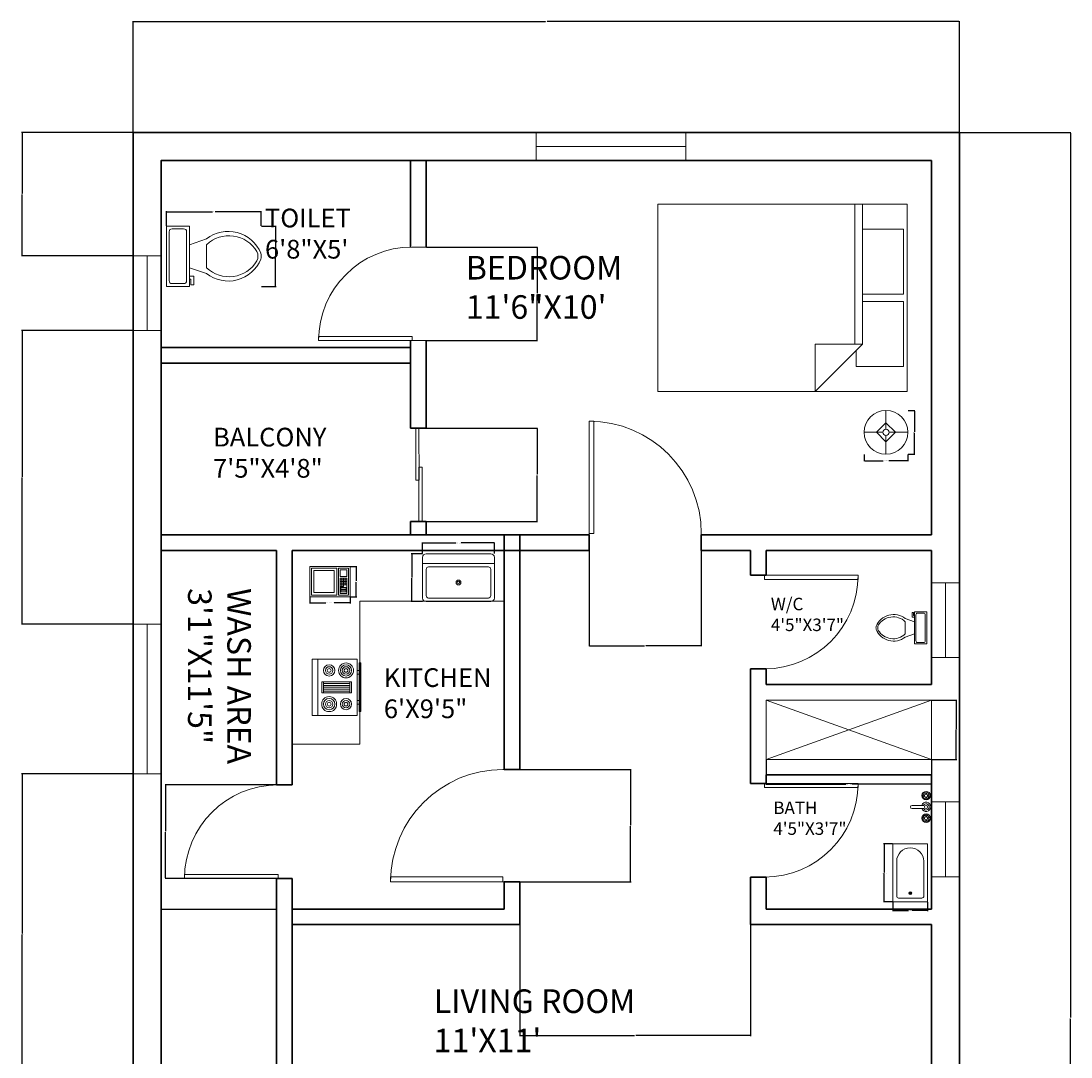
# Model space of a CAD drawing. Units: inches. Extents: x 7766 to 8631, y 9203 to 9940.
# Tile 6 of 6: x 8294 to 8631, y 9608 to 9940. Entities that reach past the tile are written whole.
import ezdxf

# ---------------------------------------------------------------- set-up
doc = ezdxf.new("R2010")
doc.units = ezdxf.units.IN
for name, color, linetype, lineweight in [('A-ANNO-DIMS', 2, 'Continuous', 18), ('A-AREA-IDEN', 11, 'Continuous', 18), ('A-EQPM', 9, 'Continuous', 18), ('A-FLOR-CASE', 7, 'Continuous', 20), ('A-FLOR-FIXT', 9, 'Continuous', 18), ('A-FLOR-OPEN', 7, 'Continuous', 18), ('A-WALL', 7, 'Continuous', 35), ('door', 1, 'Continuous', 18), ('floor', 7, 'Continuous', 25), ('furniture', 6, 'Continuous', 18), ('window', 3, 'Continuous', 18)]:
    doc.layers.add(name, color=color, linetype=linetype, lineweight=lineweight)
doc.styles.get("Standard").update_dxf_attribs({"font": 'arial.ttf'})
doc.dimstyles.get("Standard").update_dxf_attribs({"dimtxt": 0.18, "dimasz": 0.18, "dimexe": 0.18, "dimexo": 0.0625, "dimgap": 0.09, "dimtad": 0, "dimtih": 1, "dimtoh": 1, "dimdec": 4, "dimzin": 0, "dimdsep": 46, "dimtxsty": 'Standard', "dimcen": 0.09, "dimadec": 0, "dimazin": 0, "dimtfac": 1, "dimtdec": 4, "dimtofl": 0, "dimtmove": 0, "dimatfit": 3, "dimfxl": 1, "dimtolj": 1, "dimtzin": 0, "dimarcsym": 0})

# ---------------------------------------------------------------- blocks, each defined once
blk = doc.blocks.new('*U2')
for p, q in [((0, 0), (0, -6)), ((40, 0), (40, -6))]:
    blk.add_line(p, q)
blk.add_lwpolyline([(0, 0), (0, 40), (1.75, 40), (1.75, 0)], close=True)
blk.add_arc((0, 0), 40, 0, 90)
blk = doc.blocks.new('*U4')
for p, q in [((0, 0), (0, -6)), ((40, 0), (40, -6))]:
    blk.add_line(p, q)
blk.add_lwpolyline([(0, 0), (0, 40), (1.75, 40), (1.75, 0)], close=True)
blk.add_arc((0, 0), 40, 0, 90)
blk = doc.blocks.new('Bed - Queen')
for p, q in [((0, -80.00003), (0, 0)), ((0, 0), (59.99999, 0)), ((59.99999, 0), (59.99999, -80.00003)), ((7.99999, -1.2), (28.79998, -1.2)), ((7.99999, -14.4), (7.99999, -1.2)), ((28.79998, -1.2), (28.79998, -14.4)), ((31.19999, -1.2), (51.99999, -1.2)), ((31.19999, -14.4), (31.19999, -1.2)), ((51.99999, -1.2), (51.99999, -16.4)), ((0, -14.4), (44.8, -14.4)), ((44.8, -16.8), (0, -16.8)), ((59.99999, -29.6), (44.8, -14.4)), ((44.8, -14.4), (44.8, -29.6)), ((51.99999, -16.4), (46.79936, -16.4)), ((44.8, -29.6), (59.99999, -29.6)), ((59.99999, -80.00003), (0, -80.00003))]:
    blk.add_line(p, q)
blk = doc.blocks.new('Microwave')
for p, q in [((18, 10), (22, 10)), ((22, 9), (18, 9)), ((18, 8), (22, 8)), ((22, 7), (18, 7)), ((19, 7), (19, 11)), ((19, 6), (19, 7)), ((20, 11), (20, 7)), ((20, 7), (20, 6)), ((21, 7), (21, 11)), ((20, 6), (18, 6))]:
    blk.add_line(p, q)
for points in [[(0, 0), (0, 18), (24, 18), (24, 0)], [(1, 1), (1, 17), (16, 17), (16, 1)], [(2.5, 2.5), (2.5, 15.5), (14.5, 15.5), (14.5, 2.5)], [(17, 1), (17, 17), (23, 17), (23, 1)], [(18, 12), (18, 16), (22, 16), (22, 12)], [(18, 2), (18, 11), (22, 11), (22, 2)], [(18.5, 4.5), (18.5, 5.5), (21.5, 5.5), (21.5, 4.5)], [(18.5, 3), (18.5, 4), (21.5, 4), (21.5, 3)]]:
    blk.add_lwpolyline(points, close=True)
blk = doc.blocks.new('Range-Oven - 30 in top')
for p, q in [((0, -3), (30, -3)), ((12, -6), (18, -6)), ((13, -20), (13, -6)), ((14, -6), (14, -20)), ((15, -20), (15, -6)), ((16, -6), (16, -20)), ((17, -20), (17, -6)), ((18, -20), (12, -20)), ((6, -24), (6, -25)), ((8, -25), (8, -24)), ((22, -25), (22, -24)), ((24, -24), (24, -25))]:
    blk.add_line(p, q)
for points in [[(0, -24), (0, 0), (30, 0), (30, -24)], [(12, -21), (12, -5), (18, -5), (18, -21)], [(2, -26), (2, -25), (28, -25), (28, -26)]]:
    blk.add_lwpolyline(points, close=True)
for centre, radius in [((6, -9), 4), ((6, -9), 3), ((6, -9), 2), ((6, -9), 1), ((24, -9), 3), ((24, -9), 2), ((24, -9), 1), ((6, -18), 3), ((6, -18), 2), ((24, -18), 4), ((24, -18), 3), ((24, -18), 2), ((6, -18), 1), ((24, -18), 1)]:
    blk.add_circle(centre, radius)
blk = doc.blocks.new('Sink-single - 30 in top')
blk.add_line((-15, -3.999996), (15, -3.999996))
for points in [[(-13.5, 0), (13.5, 0)], [(-15, -18.499996), (-15, -1.5)], [(15, -1.5), (15, -18.499996)], [(-13.5, -17.499996), (-13.5, -6.499996)], [(-12.5, -5.499996), (12.5, -5.499996)], [(13.5, -6.499996), (13.5, -17.499996)], [(13.5, -19.999996), (-13.5, -19.999996)], [(12.5, -18.499996), (-12.5, -18.499996)]]:
    blk.add_lwpolyline(points)
for radius in [1, 0.5]:
    blk.add_circle((0, -11.999996), radius)
for centre, radius, start, end in [((-13.5, -1.5), 1.5, 90, 180), ((13.5, -1.5), 1.5, 0, 90), ((-12.5, -6.499996), 1, 90, 180), ((12.5, -6.499996), 1, 0, 90), ((-12.5, -17.499996), 1, 180, 270), ((12.5, -17.499996), 1, 270, 0), ((-13.5, -18.499996), 1.5, 180, 270), ((13.5, -18.499996), 1.5, 270, 0)]:
    blk.add_arc(centre, radius, start, end)
blk = doc.blocks.new('Lamp - Table')
for p, q in [((0, 7), (0, 1)), ((-1, 0), (-7, 0)), ((0, 3), (-3, 0)), ((-3, 0), (0, -3)), ((3, 0), (0, 3)), ((0, -3), (3, 0)), ((1, 0), (7, 0)), ((0, -1), (0, -7))]:
    blk.add_line(p, q)
for radius in [7, 1]:
    blk.add_circle((0, 0), radius)
blk = doc.blocks.new('Toilet - top')
for p, q in [((9.5, -6), (9.5, -2)), ((-10, -8.5), (-8, -8.5)), ((-10, -9.5), (-10, -8.5)), ((-7, -9.5), (-10, -9.5)), ((-8, -8.5), (-8, -8)), ((-7, -8), (-7, -9.5)), ((-4, -8), (-6, -14)), ((4, -8), (6, -14)), ((4, -14), (-4, -14))]:
    blk.add_line(p, q)
blk.add_lwpolyline([(10.5, -8), (10.5, 0), (-10.5, 0), (-10.5, -8)], close=True)
for points in [[(-9.5, -2), (-9.5, -6)], [(8.5, -1), (-8.5, -1)], [(-8.5, -7), (8.5, -7)]]:
    blk.add_lwpolyline(points)
for centre, radius, start, end in [((-8.62, -1.88), 0.884, 81.8699, 188.1301), ((8.62, -1.88), 0.884, 351.8699, 98.1301), ((-8.62, -6.12), 0.884, 171.8699, 278.1301), ((8.62, -6.12), 0.884, 261.8699, 8.1301), ((3.52, -21.58), 12.17, 141.4691, 247.9714), ((4.2, -21.82), 11.33, 136.3677, 238.9468), ((-3.52, -21.58), 12.17, 292.0284, 38.5307), ((-4.2, -21.82), 11.33, 301.053, 43.6321), ((0, -27.88), 4, 245.7318, 294.2682), ((0, -29), 4, 254.8605, 285.1395)]:
    blk.add_arc(centre, radius, start, end)
blk = doc.blocks.new('Faucet - Bathroom top')
for p, q in [((-4.107, 0.125), (-4.375, 0.125)), ((-3.75, 0.4788), (-3.75, 0.75)), ((-3.5, 0.482), (-3.5, 0.75)), ((-3.1461, 0.125), (-2.875, 0.125)), ((3.143, 0.125), (2.875, 0.125)), ((3.5, 0.4788), (3.5, 0.75)), ((3.75, 0.482), (3.75, 0.75)), ((4.1039, 0.125), (4.375, 0.125)), ((-4.1039, -0.125), (-4.375, -0.125)), ((-3.75, -0.4821), (-3.75, -0.75)), ((-3.5, -0.4789), (-3.5, -0.75)), ((-3.143, -0.125), (-2.875, -0.125)), ((-0.5, -0.8639), (-0.5, -4.5)), ((0.5, -4.5), (0.5, -0.8631)), ((3.1461, -0.125), (2.875, -0.125)), ((3.5, -0.4821), (3.5, -0.75)), ((3.75, -0.4789), (3.75, -0.75)), ((4.107, -0.125), (4.375, -0.125))]:
    blk.add_line(p, q)
for centre, radius in [((-3.625, 0), 1.375), ((-4.625, 0), 0.2795), ((-3.625, 0), 0.5), ((-3.625, 1), 0.2795), ((-2.625, 0), 0.2795), ((0, 0), 0.5), ((3.625, 0), 1.375), ((2.625, 0), 0.2795), ((3.625, 0), 0.5), ((3.625, 1), 0.2795), ((4.625, 0), 0.2795), ((-3.625, -1), 0.2795), ((3.625, -1), 0.2795)]:
    blk.add_circle(centre, radius)
for centre, radius, start, end in [((-3.625, 0), 1, 105.2407, 164.2093), ((-3.625, 0), 1, 16.44125, 74.07887), ((0, 0), 1.5, 289.6514, 250.3603), ((0, 0), 1, 300.3431, 239.7554), ((3.625, 0), 1, 106.12, 164.0884), ((3.625, 0), 1, 16.23422, 73.90469), ((-3.625, 0), 1, 196.2342, 253.9047), ((-3.625, 0), 1, 286.12, 344.0884), ((3.625, 0), 1, 196.4413, 254.0789), ((3.625, 0), 1, 285.2407, 344.2093), ((0, -4.5), 0.5, 180, 0)]:
    blk.add_arc(centre, radius, start, end)
blk = doc.blocks.new('Bath Tub - 26 x 60 in.')
for p, q in [((8, -18), (10, -18)), ((9, -17), (9, -19))]:
    blk.add_line(p, q)
blk.add_lwpolyline([(0, -36), (0, 0), (60, 0), (60, -36)], close=True)
for points in [[(4, -30), (4, -6)], [(6, -4), (42, -4)], [(42, -32), (6, -32)]]:
    blk.add_lwpolyline(points)
for radius in [1.5, 1]:
    blk.add_circle((9, -18), radius)
for centre, radius, start, end in [((5.75, -5.75), 1.77, 81.8699, 188.1301), ((42, -18), 14, 270, 90), ((5.75, -30.25), 1.77, 171.8699, 278.1301)]:
    blk.add_arc(centre, radius, start, end)
blk = doc.blocks.new('WIN-48IN')
blk.add_line((4.5, 48), (4.5, 0))
blk.add_lwpolyline([(0, 48), (9, 48), (9, 0), (0, 0)], close=True)
blk = doc.blocks.new('WIN-24IN')
blk.add_line((4.5, 24), (4.5, 0))
blk.add_lwpolyline([(0, 24), (9, 24), (9, 0), (0, 0)], close=True)
blk = doc.blocks.new('COUNTER-L-KITCHEN')
for points in [[(21.71, 45.84), (68, 45.84), (68, 62.12), (0, 62.12), (0, 45.84)], [(21.71, 45.84), (21.71, 0), (0, 0), (0, 62.12), (21.71, 62.12)]]:
    blk.add_lwpolyline(points)
blk = doc.blocks.new('SHAFT-53X19')
for p, q in [((0, 19), (53, 19)), ((0, 0), (0, 19)), ((0, 19), (53, 0)), ((53, 19), (0, 0)), ((53, 0), (53, 19)), ((0, 0), (53, 0))]:
    blk.add_line(p, q)
blk = doc.blocks.new('*D34')
at = {"layer": 'A-ANNO-DIMS', "color": 0, "lineweight": -2, "transparency": 16777216}
for p, q in [((8340.53, 9874.62), (8340.53, 9879.3)), ((8340.71, 9879.12), (8355.28, 9879.12)), ((8370.78, 9879.12), (8356.21, 9879.12)), ((8370.96, 9874.62), (8370.96, 9879.3))]:
    blk.add_line(p, q, dxfattribs=at)
at = {"layer": 'A-ANNO-DIMS', "color": 0, "transparency": 16777216}
for points in [[(8340.71, 9879.15), (8340.71, 9879.09), (8340.53, 9879.12)], [(8370.78, 9879.15), (8370.78, 9879.09), (8370.96, 9879.12)]]:
    blk.add_solid(points, dxfattribs=at)
at = {"layer": 'Defpoints', "color": 0, "transparency": 16777216}
for p in [(8340.53, 9879.12), (8340.53, 9874.55), (8370.96, 9874.55)]:
    blk.add_point(p, dxfattribs=at)
at = {"layer": 'A-ANNO-DIMS', "color": 0, "transparency": 16777216, "insert": (8355.75, 9879.12), "char_height": 0.18, "attachment_point": 5}
blk.add_mtext('\\A1;WC 30', dxfattribs=at)
blk = doc.blocks.new('*D35')
at = {"layer": 'A-ANNO-DIMS', "color": 0, "lineweight": -2, "transparency": 16777216}
for p, q in [((8371.03, 9874.55), (8375.71, 9874.55)), ((8375.53, 9874.37), (8375.53, 9865.07)), ((8375.53, 9855.39), (8375.53, 9864.7)), ((8371.03, 9855.21), (8375.71, 9855.21))]:
    blk.add_line(p, q, dxfattribs=at)
at = {"layer": 'A-ANNO-DIMS', "color": 0, "transparency": 16777216}
for points in [[(8375.5, 9874.37), (8375.56, 9874.37), (8375.53, 9874.55)], [(8375.5, 9855.39), (8375.56, 9855.39), (8375.53, 9855.21)]]:
    blk.add_solid(points, dxfattribs=at)
at = {"layer": 'Defpoints', "color": 0, "transparency": 16777216}
for p in [(8370.96, 9874.55), (8375.53, 9874.55), (8370.96, 9855.21)]:
    blk.add_point(p, dxfattribs=at)
at = {"layer": 'A-ANNO-DIMS', "color": 0, "transparency": 16777216, "insert": (8375.53, 9864.88), "char_height": 0.18, "attachment_point": 5}
blk.add_mtext('\\A1;19', dxfattribs=at)
blk = doc.blocks.new('*D46')
at = {"layer": 'A-ANNO-DIMS', "color": 0, "lineweight": -2, "transparency": 16777216}
for p, q in [((8386.48, 9755.63), (8386.48, 9753.56)), ((8386.66, 9753.74), (8391.63, 9753.74)), ((8399.3, 9753.74), (8394.33, 9753.74)), ((8399.48, 9755.63), (8399.48, 9753.56))]:
    blk.add_line(p, q, dxfattribs=at)
at = {"layer": 'A-ANNO-DIMS', "color": 0, "transparency": 16777216}
for points in [[(8386.66, 9753.77), (8386.66, 9753.71), (8386.48, 9753.74)], [(8399.3, 9753.77), (8399.3, 9753.71), (8399.48, 9753.74)]]:
    blk.add_solid(points, dxfattribs=at)
at = {"layer": 'Defpoints', "color": 0, "transparency": 16777216}
for p in [(8386.48, 9755.69), (8399.48, 9755.69), (8399.48, 9753.74)]:
    blk.add_point(p, dxfattribs=at)
at = {"layer": 'A-ANNO-DIMS', "color": 0, "transparency": 16777216, "insert": (8392.98, 9753.74), "char_height": 0.18, "attachment_point": 5}
blk.add_mtext('\\A1;MICROWAVE 13 TYP.', dxfattribs=at)
blk = doc.blocks.new('*D47')
at = {"layer": 'A-ANNO-DIMS', "color": 0, "lineweight": -2, "transparency": 16777216}
for p, q in [((8399.54, 9765.44), (8401.61, 9765.44)), ((8401.43, 9765.26), (8401.43, 9760.75)), ((8401.43, 9755.87), (8401.43, 9760.38)), ((8399.54, 9755.69), (8401.61, 9755.69))]:
    blk.add_line(p, q, dxfattribs=at)
at = {"layer": 'A-ANNO-DIMS', "color": 0, "transparency": 16777216}
for points in [[(8401.4, 9765.26), (8401.46, 9765.26), (8401.43, 9765.44)], [(8401.4, 9755.87), (8401.46, 9755.87), (8401.43, 9755.69)]]:
    blk.add_solid(points, dxfattribs=at)
at = {"layer": 'Defpoints', "color": 0, "transparency": 16777216}
for p in [(8399.48, 9765.44), (8401.43, 9765.44), (8399.48, 9755.69)]:
    blk.add_point(p, dxfattribs=at)
at = {"layer": 'A-ANNO-DIMS', "color": 0, "transparency": 16777216, "insert": (8401.43, 9760.56), "char_height": 0.18, "attachment_point": 5}
blk.add_mtext('\\A1;10 TYP.', dxfattribs=at)
blk = doc.blocks.new('*D50')
at = {"layer": 'A-ANNO-DIMS', "color": 0, "lineweight": -2, "transparency": 16777216}
for p, q in [((8422.69, 9769.54), (8422.69, 9773.11)), ((8422.87, 9772.93), (8433.33, 9772.93)), ((8445.51, 9772.93), (8435.04, 9772.93)), ((8445.69, 9769.54), (8445.69, 9773.11))]:
    blk.add_line(p, q, dxfattribs=at)
at = {"layer": 'A-ANNO-DIMS', "color": 0, "transparency": 16777216}
for points in [[(8422.87, 9772.96), (8422.87, 9772.9), (8422.69, 9772.93)], [(8445.51, 9772.96), (8445.51, 9772.9), (8445.69, 9772.93)]]:
    blk.add_solid(points, dxfattribs=at)
at = {"layer": 'Defpoints', "color": 0, "transparency": 16777216}
for p in [(8445.69, 9772.93), (8422.69, 9769.48), (8445.69, 9769.48)]:
    blk.add_point(p, dxfattribs=at)
at = {"layer": 'A-ANNO-DIMS', "color": 0, "transparency": 16777216, "insert": (8434.19, 9772.93), "char_height": 0.18, "attachment_point": 5}
blk.add_mtext('\\A1;SINK 23 TYP.', dxfattribs=at)
blk = doc.blocks.new('*D51')
at = {"layer": 'A-ANNO-DIMS', "color": 0, "lineweight": -2, "transparency": 16777216}
for p, q in [((8422.62, 9769.48), (8419.06, 9769.48)), ((8419.24, 9769.3), (8419.24, 9761.99)), ((8419.24, 9754.32), (8419.24, 9761.63)), ((8422.62, 9754.14), (8419.06, 9754.14))]:
    blk.add_line(p, q, dxfattribs=at)
at = {"layer": 'A-ANNO-DIMS', "color": 0, "transparency": 16777216}
for points in [[(8419.21, 9769.3), (8419.27, 9769.3), (8419.24, 9769.48)], [(8419.21, 9754.32), (8419.27, 9754.32), (8419.24, 9754.14)]]:
    blk.add_solid(points, dxfattribs=at)
at = {"layer": 'Defpoints', "color": 0, "transparency": 16777216}
for p in [(8419.24, 9769.48), (8422.69, 9769.48), (8422.69, 9754.14)]:
    blk.add_point(p, dxfattribs=at)
at = {"layer": 'A-ANNO-DIMS', "color": 0, "transparency": 16777216, "insert": (8419.24, 9761.81), "char_height": 0.18, "attachment_point": 5}
blk.add_mtext('\\A1;15 TYP.', dxfattribs=at)
blk = doc.blocks.new('*D52')
at = {"layer": 'A-ANNO-DIMS', "color": 0, "lineweight": -2, "transparency": 16777216}
for p, q in [((8564.27, 9801.35), (8564.27, 9799.13)), ((8578.27, 9801.35), (8578.27, 9799.13)), ((8564.45, 9799.31), (8570.37, 9799.31)), ((8578.09, 9799.31), (8572.17, 9799.31))]:
    blk.add_line(p, q, dxfattribs=at)
at = {"layer": 'A-ANNO-DIMS', "color": 0, "transparency": 16777216}
for points in [[(8564.45, 9799.34), (8564.45, 9799.28), (8564.27, 9799.31)], [(8578.09, 9799.34), (8578.09, 9799.28), (8578.27, 9799.31)]]:
    blk.add_solid(points, dxfattribs=at)
at = {"layer": 'Defpoints', "color": 0, "transparency": 16777216}
for p in [(8564.27, 9801.41), (8578.27, 9801.41), (8578.27, 9799.31)]:
    blk.add_point(p, dxfattribs=at)
at = {"layer": 'A-ANNO-DIMS', "color": 0, "transparency": 16777216, "insert": (8571.27, 9799.31), "char_height": 0.18, "attachment_point": 5}
blk.add_mtext('\\A1;LAMP 14 TYP.', dxfattribs=at)
blk = doc.blocks.new('*D53')
at = {"layer": 'A-ANNO-DIMS', "color": 0, "lineweight": -2, "transparency": 16777216}
for p, q in [((8578.33, 9815.41), (8580.55, 9815.41)), ((8580.37, 9815.23), (8580.37, 9808.59)), ((8580.37, 9801.59), (8580.37, 9808.23)), ((8578.33, 9801.41), (8580.55, 9801.41))]:
    blk.add_line(p, q, dxfattribs=at)
at = {"layer": 'A-ANNO-DIMS', "color": 0, "transparency": 16777216}
for points in [[(8580.34, 9815.23), (8580.4, 9815.23), (8580.37, 9815.41)], [(8580.34, 9801.59), (8580.4, 9801.59), (8580.37, 9801.41)]]:
    blk.add_solid(points, dxfattribs=at)
at = {"layer": 'Defpoints', "color": 0, "transparency": 16777216}
for p in [(8578.27, 9815.41), (8580.37, 9815.41), (8578.27, 9801.41)]:
    blk.add_point(p, dxfattribs=at)
at = {"layer": 'A-ANNO-DIMS', "color": 0, "transparency": 16777216, "insert": (8580.37, 9808.41), "char_height": 0.18, "attachment_point": 5}
blk.add_mtext('\\A1;14 TYP.', dxfattribs=at)
blk = doc.blocks.new('*D56')
at = {"layer": 'A-ANNO-DIMS', "color": 0, "lineweight": -2, "transparency": 16777216}
for p, q in [((8573.4, 9676.45), (8570.49, 9676.45)), ((8570.67, 9676.27), (8570.67, 9667.33)), ((8570.67, 9658.03), (8570.67, 9666.97)), ((8573.4, 9657.85), (8570.49, 9657.85))]:
    blk.add_line(p, q, dxfattribs=at)
at = {"layer": 'A-ANNO-DIMS', "color": 0, "transparency": 16777216}
for points in [[(8570.64, 9676.27), (8570.7, 9676.27), (8570.67, 9676.45)], [(8570.64, 9658.03), (8570.7, 9658.03), (8570.67, 9657.85)]]:
    blk.add_solid(points, dxfattribs=at)
at = {"layer": 'Defpoints', "color": 0, "transparency": 16777216}
for p in [(8570.67, 9676.45), (8573.46, 9676.45), (8573.46, 9657.85)]:
    blk.add_point(p, dxfattribs=at)
at = {"layer": 'A-ANNO-DIMS', "color": 0, "transparency": 16777216, "insert": (8570.67, 9667.15), "char_height": 0.18, "attachment_point": 5}
blk.add_mtext('\\A1;TUB 19 TYP.', dxfattribs=at)
blk = doc.blocks.new('*D57')
at = {"layer": 'A-ANNO-DIMS', "color": 0, "lineweight": -2, "transparency": 16777216}
for p, q in [((8573.46, 9657.79), (8573.46, 9654.88)), ((8584.62, 9657.79), (8584.62, 9654.88)), ((8573.64, 9655.06), (8578.52, 9655.06)), ((8584.44, 9655.06), (8579.56, 9655.06))]:
    blk.add_line(p, q, dxfattribs=at)
at = {"layer": 'A-ANNO-DIMS', "color": 0, "transparency": 16777216}
for points in [[(8573.64, 9655.09), (8573.64, 9655.03), (8573.46, 9655.06)], [(8584.44, 9655.09), (8584.44, 9655.03), (8584.62, 9655.06)]]:
    blk.add_solid(points, dxfattribs=at)
at = {"layer": 'Defpoints', "color": 0, "transparency": 16777216}
for p in [(8573.46, 9657.85), (8584.62, 9657.85), (8573.46, 9655.06)]:
    blk.add_point(p, dxfattribs=at)
at = {"layer": 'A-ANNO-DIMS', "color": 0, "transparency": 16777216, "insert": (8579.04, 9655.06), "char_height": 0.18, "attachment_point": 5}
blk.add_mtext('\\A1;11 TYP.', dxfattribs=at)
blk = doc.blocks.new('*D64')
at = {"layer": 'A-ANNO-DIMS', "color": 0, "lineweight": -2, "transparency": 16777216}
for p, q in [((8532.84, 9703.5), (8532.84, 9695.43)), ((8585.84, 9703.5), (8585.84, 9695.43)), ((8533.02, 9695.61), (8558.36, 9695.61)), ((8585.66, 9695.61), (8560.31, 9695.61))]:
    blk.add_line(p, q, dxfattribs=at)
at = {"layer": 'A-ANNO-DIMS', "color": 0, "transparency": 16777216}
for points in [[(8533.02, 9695.64), (8533.02, 9695.58), (8532.84, 9695.61)], [(8585.66, 9695.64), (8585.66, 9695.58), (8585.84, 9695.61)]]:
    blk.add_solid(points, dxfattribs=at)
at = {"layer": 'Defpoints', "color": 0, "transparency": 16777216}
for p in [(8532.84, 9703.56), (8585.84, 9703.56), (8532.84, 9695.61)]:
    blk.add_point(p, dxfattribs=at)
at = {"layer": 'A-ANNO-DIMS', "color": 0, "transparency": 16777216, "insert": (8559.34, 9695.61), "char_height": 0.18, "attachment_point": 5}
blk.add_mtext('\\A1;SHAFT 53 TYP.', dxfattribs=at)
blk = doc.blocks.new('*D65')
at = {"layer": 'A-ANNO-DIMS', "color": 0, "lineweight": -2, "transparency": 16777216}
for p, q in [((8585.9, 9722.56), (8593.97, 9722.56)), ((8593.79, 9722.38), (8593.79, 9713.25)), ((8593.79, 9703.74), (8593.79, 9712.88)), ((8585.9, 9703.56), (8593.97, 9703.56))]:
    blk.add_line(p, q, dxfattribs=at)
at = {"layer": 'A-ANNO-DIMS', "color": 0, "transparency": 16777216}
for points in [[(8593.76, 9722.38), (8593.82, 9722.38), (8593.79, 9722.56)], [(8593.76, 9703.74), (8593.82, 9703.74), (8593.79, 9703.56)]]:
    blk.add_solid(points, dxfattribs=at)
at = {"layer": 'Defpoints', "color": 0, "transparency": 16777216}
for p in [(8585.84, 9722.56), (8585.84, 9703.56), (8593.79, 9703.56)]:
    blk.add_point(p, dxfattribs=at)
at = {"layer": 'A-ANNO-DIMS', "color": 0, "transparency": 16777216, "insert": (8593.79, 9713.06), "char_height": 0.18, "attachment_point": 5}
blk.add_mtext('\\A1;19 TYP.', dxfattribs=at)
blk = doc.blocks.new('*D70')
at = {"layer": 'A-ANNO-DIMS', "color": 0, "lineweight": -2, "transparency": 16777216}
for p, q in [((8329.84, 9904.63), (8329.84, 9940.29)), ((8330.02, 9940.11), (8462.05, 9940.11)), ((8594.66, 9940.11), (8462.63, 9940.11)), ((8594.84, 9904.63), (8594.84, 9940.29))]:
    blk.add_line(p, q, dxfattribs=at)
at = {"layer": 'A-ANNO-DIMS', "color": 0, "transparency": 16777216}
for points in [[(8330.02, 9940.14), (8330.02, 9940.08), (8329.84, 9940.11)], [(8594.66, 9940.14), (8594.66, 9940.08), (8594.84, 9940.11)]]:
    blk.add_solid(points, dxfattribs=at)
at = {"layer": 'Defpoints', "color": 0, "transparency": 16777216}
for p in [(8594.84, 9940.11), (8329.84, 9904.56), (8594.84, 9904.56)]:
    blk.add_point(p, dxfattribs=at)
at = {"layer": 'A-ANNO-DIMS', "color": 0, "transparency": 16777216, "insert": (8462.34, 9940.11), "char_height": 0.18, "attachment_point": 5}
blk.add_mtext('\\A1;265', dxfattribs=at)
blk = doc.blocks.new('*D71')
at = {"layer": 'A-ANNO-DIMS', "color": 0, "lineweight": -2, "transparency": 16777216}
for p, q in [((8594.9, 9904.56), (8630.57, 9904.56)), ((8630.39, 9904.38), (8630.39, 9620.75)), ((8630.39, 9336.74), (8630.39, 9620.38)), ((8466.9, 9336.56), (8630.57, 9336.56))]:
    blk.add_line(p, q, dxfattribs=at)
at = {"layer": 'A-ANNO-DIMS', "color": 0, "transparency": 16777216}
for points in [[(8630.36, 9904.38), (8630.42, 9904.38), (8630.39, 9904.56)], [(8630.36, 9336.74), (8630.42, 9336.74), (8630.39, 9336.56)]]:
    blk.add_solid(points, dxfattribs=at)
at = {"layer": 'Defpoints', "color": 0, "transparency": 16777216}
for p in [(8594.84, 9904.56), (8630.39, 9904.56), (8466.84, 9336.56)]:
    blk.add_point(p, dxfattribs=at)
at = {"layer": 'A-ANNO-DIMS', "color": 0, "transparency": 16777216, "insert": (8630.39, 9620.56), "char_height": 0.18, "attachment_point": 5}
blk.add_mtext('\\A1;568', dxfattribs=at)
blk = doc.blocks.new('*D77')
at = {"layer": 'A-ANNO-DIMS', "color": 0, "lineweight": -2, "transparency": 16777216}
for p, q in [((8329.77, 9904.56), (8294.11, 9904.56)), ((8294.29, 9904.38), (8294.29, 9884.99)), ((8294.29, 9865.23), (8294.29, 9884.63)), ((8329.77, 9865.05), (8294.11, 9865.05))]:
    blk.add_line(p, q, dxfattribs=at)
at = {"layer": 'A-ANNO-DIMS', "color": 0, "transparency": 16777216}
for points in [[(8294.26, 9904.38), (8294.32, 9904.38), (8294.29, 9904.56)], [(8294.26, 9865.23), (8294.32, 9865.23), (8294.29, 9865.05)]]:
    blk.add_solid(points, dxfattribs=at)
at = {"layer": 'Defpoints', "color": 0, "transparency": 16777216}
for p in [(8294.29, 9904.56), (8329.84, 9904.56), (8329.84, 9865.05)]:
    blk.add_point(p, dxfattribs=at)
at = {"layer": 'A-ANNO-DIMS', "color": 0, "transparency": 16777216, "insert": (8294.29, 9884.81), "char_height": 0.18, "attachment_point": 5}
blk.add_mtext('\\A1;39.51', dxfattribs=at)
blk = doc.blocks.new('*D78')
at = {"layer": 'A-ANNO-DIMS', "color": 0, "lineweight": -2, "transparency": 16777216}
for p, q in [((8329.77, 9841.05), (8294.11, 9841.05)), ((8294.29, 9840.87), (8294.29, 9794.17)), ((8294.29, 9747.1), (8294.29, 9793.8)), ((8329.77, 9746.92), (8294.11, 9746.92))]:
    blk.add_line(p, q, dxfattribs=at)
at = {"layer": 'A-ANNO-DIMS', "color": 0, "transparency": 16777216}
for points in [[(8294.26, 9840.87), (8294.32, 9840.87), (8294.29, 9841.05)], [(8294.26, 9747.1), (8294.32, 9747.1), (8294.29, 9746.92)]]:
    blk.add_solid(points, dxfattribs=at)
at = {"layer": 'Defpoints', "color": 0, "transparency": 16777216}
for p in [(8294.29, 9841.05), (8329.84, 9841.05), (8329.84, 9746.92)]:
    blk.add_point(p, dxfattribs=at)
at = {"layer": 'A-ANNO-DIMS', "color": 0, "transparency": 16777216, "insert": (8294.29, 9793.99), "char_height": 0.18, "attachment_point": 5}
blk.add_mtext('\\A1;94.13', dxfattribs=at)
blk = doc.blocks.new('*D79')
at = {"layer": 'A-ANNO-DIMS', "color": 0, "lineweight": -2, "transparency": 16777216}
for p, q in [((8329.77, 9698.92), (8294.11, 9698.92)), ((8294.29, 9698.74), (8294.29, 9647.76)), ((8294.29, 9596.42), (8294.29, 9647.4)), ((8329.77, 9596.24), (8294.11, 9596.24))]:
    blk.add_line(p, q, dxfattribs=at)
at = {"layer": 'A-ANNO-DIMS', "color": 0, "transparency": 16777216}
for points in [[(8294.26, 9698.74), (8294.32, 9698.74), (8294.29, 9698.92)], [(8294.26, 9596.42), (8294.32, 9596.42), (8294.29, 9596.24)]]:
    blk.add_solid(points, dxfattribs=at)
at = {"layer": 'Defpoints', "color": 0, "transparency": 16777216}
for p in [(8294.29, 9698.92), (8329.84, 9698.92), (8329.84, 9596.24)]:
    blk.add_point(p, dxfattribs=at)
at = {"layer": 'A-ANNO-DIMS', "color": 0, "transparency": 16777216, "insert": (8294.29, 9647.58), "char_height": 0.18, "attachment_point": 5}
blk.add_mtext('\\A1;102.69', dxfattribs=at)
blk = doc.blocks.new('*D90')
at = {"layer": 'A-ANNO-DIMS', "color": 0, "lineweight": -2, "transparency": 16777216}
for p, q in [((8476.05, 9775.5), (8476.05, 9739.83)), ((8512.05, 9775.5), (8512.05, 9739.83)), ((8476.23, 9740.01), (8493.83, 9740.01)), ((8511.87, 9740.01), (8494.27, 9740.01))]:
    blk.add_line(p, q, dxfattribs=at)
at = {"layer": 'A-ANNO-DIMS', "color": 0, "transparency": 16777216}
for points in [[(8476.23, 9740.04), (8476.23, 9739.98), (8476.05, 9740.01)], [(8511.87, 9740.04), (8511.87, 9739.98), (8512.05, 9740.01)]]:
    blk.add_solid(points, dxfattribs=at)
at = {"layer": 'Defpoints', "color": 0, "transparency": 16777216}
for p in [(8476.05, 9775.56), (8512.05, 9775.56), (8476.05, 9740.01)]:
    blk.add_point(p, dxfattribs=at)
at = {"layer": 'A-ANNO-DIMS', "color": 0, "transparency": 16777216, "insert": (8494.05, 9740.01), "char_height": 0.18, "attachment_point": 5}
blk.add_mtext('\\A1;36', dxfattribs=at)
blk = doc.blocks.new('*D95')
at = {"layer": 'A-ANNO-DIMS', "color": 0, "lineweight": -2, "transparency": 16777216}
for p, q in [((8453.9, 9700.31), (8489.57, 9700.31)), ((8489.39, 9700.13), (8489.39, 9682.49)), ((8489.39, 9664.49), (8489.39, 9682.13)), ((8453.9, 9664.31), (8489.57, 9664.31))]:
    blk.add_line(p, q, dxfattribs=at)
at = {"layer": 'A-ANNO-DIMS', "color": 0, "transparency": 16777216}
for points in [[(8489.36, 9700.13), (8489.42, 9700.13), (8489.39, 9700.31)], [(8489.36, 9664.49), (8489.42, 9664.49), (8489.39, 9664.31)]]:
    blk.add_solid(points, dxfattribs=at)
at = {"layer": 'Defpoints', "color": 0, "transparency": 16777216}
for p in [(8453.84, 9700.31), (8453.84, 9664.31), (8489.39, 9664.31)]:
    blk.add_point(p, dxfattribs=at)
at = {"layer": 'A-ANNO-DIMS', "color": 0, "transparency": 16777216, "insert": (8489.39, 9682.31), "char_height": 0.18, "attachment_point": 5}
blk.add_mtext('\\A1;36', dxfattribs=at)
blk = doc.blocks.new('*D96')
at = {"layer": 'A-ANNO-DIMS', "color": 0, "lineweight": -2, "transparency": 16777216}
for p, q in [((8375.77, 9695.36), (8340.11, 9695.36)), ((8340.29, 9695.18), (8340.29, 9680.54)), ((8340.29, 9665.54), (8340.29, 9680.18)), ((8375.77, 9665.36), (8340.11, 9665.36))]:
    blk.add_line(p, q, dxfattribs=at)
at = {"layer": 'A-ANNO-DIMS', "color": 0, "transparency": 16777216}
for points in [[(8340.26, 9695.18), (8340.32, 9695.18), (8340.29, 9695.36)], [(8340.26, 9665.54), (8340.32, 9665.54), (8340.29, 9665.36)]]:
    blk.add_solid(points, dxfattribs=at)
at = {"layer": 'Defpoints', "color": 0, "transparency": 16777216}
for p in [(8340.29, 9695.36), (8375.84, 9695.36), (8375.84, 9665.36)]:
    blk.add_point(p, dxfattribs=at)
at = {"layer": 'A-ANNO-DIMS', "color": 0, "transparency": 16777216, "insert": (8340.29, 9680.36), "char_height": 0.18, "attachment_point": 5}
blk.add_mtext('\\A1;30', dxfattribs=at)
blk = doc.blocks.new('*D97')
at = {"layer": 'A-ANNO-DIMS', "color": 0, "lineweight": -2, "transparency": 16777216}
for p, q in [((8453.84, 9650.5), (8453.84, 9614.83)), ((8527.84, 9650.5), (8527.84, 9614.83)), ((8454.02, 9615.01), (8490.62, 9615.01)), ((8527.66, 9615.01), (8491.05, 9615.01))]:
    blk.add_line(p, q, dxfattribs=at)
at = {"layer": 'A-ANNO-DIMS', "color": 0, "transparency": 16777216}
for points in [[(8454.02, 9615.04), (8454.02, 9614.98), (8453.84, 9615.01)], [(8527.66, 9615.04), (8527.66, 9614.98), (8527.84, 9615.01)]]:
    blk.add_solid(points, dxfattribs=at)
at = {"layer": 'Defpoints', "color": 0, "transparency": 16777216}
for p in [(8453.84, 9650.56), (8527.84, 9650.56), (8453.84, 9615.01)]:
    blk.add_point(p, dxfattribs=at)
at = {"layer": 'A-ANNO-DIMS', "color": 0, "transparency": 16777216, "insert": (8490.84, 9615.01), "char_height": 0.18, "attachment_point": 5}
blk.add_mtext('\\A1;74', dxfattribs=at)
blk = doc.blocks.new('*D98')
at = {"layer": 'A-ANNO-DIMS', "color": 0, "lineweight": -2, "transparency": 16777216}
for p, q in [((8423.9, 9867.83), (8459.57, 9867.83)), ((8459.39, 9867.65), (8459.39, 9853.01)), ((8459.39, 9838.01), (8459.39, 9852.65)), ((8423.9, 9837.83), (8459.57, 9837.83))]:
    blk.add_line(p, q, dxfattribs=at)
at = {"layer": 'A-ANNO-DIMS', "color": 0, "transparency": 16777216}
for points in [[(8459.36, 9867.65), (8459.42, 9867.65), (8459.39, 9867.83)], [(8459.36, 9838.01), (8459.42, 9838.01), (8459.39, 9837.83)]]:
    blk.add_solid(points, dxfattribs=at)
at = {"layer": 'Defpoints', "color": 0, "transparency": 16777216}
for p in [(8423.84, 9867.83), (8423.84, 9837.83), (8459.39, 9837.83)]:
    blk.add_point(p, dxfattribs=at)
at = {"layer": 'A-ANNO-DIMS', "color": 0, "transparency": 16777216, "insert": (8459.39, 9852.83), "char_height": 0.18, "attachment_point": 5}
blk.add_mtext('\\A1;30', dxfattribs=at)
blk = doc.blocks.new('*D99')
at = {"layer": 'A-ANNO-DIMS', "color": 0, "lineweight": -2, "transparency": 16777216}
for p, q in [((8423.9, 9809.77), (8459.57, 9809.77)), ((8459.39, 9809.59), (8459.39, 9794.95)), ((8459.39, 9779.95), (8459.39, 9794.59)), ((8423.9, 9779.77), (8459.57, 9779.77))]:
    blk.add_line(p, q, dxfattribs=at)
at = {"layer": 'A-ANNO-DIMS', "color": 0, "transparency": 16777216}
for points in [[(8459.36, 9809.59), (8459.42, 9809.59), (8459.39, 9809.77)], [(8459.36, 9779.95), (8459.42, 9779.95), (8459.39, 9779.77)]]:
    blk.add_solid(points, dxfattribs=at)
at = {"layer": 'Defpoints', "color": 0, "transparency": 16777216}
for p in [(8423.84, 9809.77), (8423.84, 9779.77), (8459.39, 9779.77)]:
    blk.add_point(p, dxfattribs=at)
at = {"layer": 'A-ANNO-DIMS', "color": 0, "transparency": 16777216, "insert": (8459.39, 9794.77), "char_height": 0.18, "attachment_point": 5}
blk.add_mtext('\\A1;30', dxfattribs=at)

msp = doc.modelspace()

# ---------------------------------------------------------------- linework, layer by layer
at = {"layer": 'A-WALL'}
for p, q in [((8329.8366, 9336.5631), (8329.8366, 9904.5631)), ((8329.8366, 9904.5631), (8594.8366, 9904.5631)), ((8594.8366, 9895.5631), (8594.8366, 9904.5631)), ((8338.8366, 9509.5631), (8338.8366, 9895.5631)), ((8338.8366, 9895.5631), (8585.8366, 9895.5631)), ((8585.8366, 9775.5631), (8585.8366, 9895.5631)), ((8594.8366, 9895.5631), (8594.8366, 9372.5631)), ((8338.8366, 9835.5631), (8418.8366, 9835.5631)), ((8338.8366, 9830.5631), (8418.8366, 9830.5631)), ((8423.8366, 9809.7709), (8418.8366, 9809.7709)), ((8423.8366, 9779.7709), (8418.8366, 9779.7709)), ((8338.8366, 9775.5631), (8476.0478, 9775.5631)), ((8448.8366, 9700.3108), (8448.8366, 9775.5631)), ((8453.8366, 9700.3108), (8453.8366, 9775.5631)), ((8512.0478, 9775.5631), (8527.8366, 9775.5631)), ((8527.8366, 9775.5631), (8585.8366, 9775.5631)), ((8375.8366, 9770.5631), (8338.8366, 9770.5631)), ((8375.8366, 9695.3613), (8375.8366, 9770.5631)), ((8380.8366, 9695.3613), (8380.8366, 9770.5631)), ((8380.8366, 9770.5631), (8476.0478, 9770.5631)), ((8512.0478, 9770.5631), (8527.8366, 9770.5631)), ((8527.8366, 9762.5783), (8527.8366, 9770.5631)), ((8532.8366, 9762.5783), (8532.8366, 9770.5631)), ((8532.8366, 9770.5631), (8585.8366, 9770.5631)), ((8585.8366, 9727.5631), (8585.8366, 9770.5631)), ((8527.8366, 9695.831), (8527.8366, 9732.5783)), ((8532.8366, 9727.5631), (8532.8366, 9732.5783)), ((8532.8366, 9727.5631), (8585.8366, 9727.5631)), ((8532.8366, 9695.831), (8532.8366, 9698.5631)), ((8532.8366, 9698.5631), (8585.8366, 9698.5631)), ((8585.8366, 9655.5631), (8585.8366, 9698.5631)), ((8375.8366, 9509.5631), (8375.8366, 9665.3613)), ((8380.8366, 9518.5631), (8380.8366, 9665.3613)), ((8448.8366, 9655.5631), (8448.8366, 9664.3108)), ((8453.8366, 9650.5631), (8453.8366, 9664.3108)), ((8527.8366, 9650.5631), (8527.8366, 9665.831)), ((8532.8366, 9655.5631), (8532.8366, 9665.831)), ((8380.8366, 9655.5631), (8448.8366, 9655.5631)), ((8380.8366, 9655.5631), (8448.8366, 9655.5631)), ((8532.8366, 9655.5631), (8585.8366, 9655.5631)), ((8380.8366, 9650.5631), (8453.8366, 9650.5631)), ((8527.8366, 9650.5631), (8585.8366, 9650.5631)), ((8585.8366, 9518.5631), (8585.8366, 9650.5631))]:
    msp.add_line(p, q, dxfattribs=at)
for points in [[(8338.8366, 9784.5631), (8338.8366, 9895.5631), (8375.8366, 9895.5631)], [(8418.8366, 9867.8266), (8418.8366, 9895.5631)], [(8423.8366, 9867.8308), (8423.8366, 9895.5631)], [(8418.8366, 9809.7667), (8418.8366, 9837.8308)], [(8423.8366, 9809.7709), (8423.8366, 9837.8308)], [(8418.8366, 9775.5631), (8418.8366, 9779.7709)], [(8423.8366, 9775.5631), (8423.8366, 9779.7709)], [(8476.0478, 9770.5631), (8476.0478, 9775.5631)], [(8512.0478, 9775.5631), (8512.0478, 9770.5631)], [(8527.8366, 9762.5783), (8532.8366, 9762.5783)], [(8532.8366, 9732.5783), (8527.8366, 9732.5783)], [(8448.8366, 9700.3108), (8453.8366, 9700.3108)], [(8375.8366, 9695.3613), (8380.8366, 9695.3613)], [(8527.8366, 9695.831), (8532.8366, 9695.831)], [(8380.8366, 9665.3613), (8375.8366, 9665.3613)], [(8453.8366, 9664.3108), (8448.8366, 9664.3108)], [(8532.8366, 9665.831), (8527.8366, 9665.831)]]:
    msp.add_lwpolyline(points, dxfattribs=at)
at = {"layer": 'door'}
for points in [[(8420.4646, 9809.7375), (8421.492, 9809.7375), (8421.5389, 9793.1278), (8420.5114, 9793.1278)], [(8421.4789, 9797.259), (8422.5064, 9797.259), (8422.5359, 9779.7709), (8421.5084, 9779.7709)]]:
    msp.add_lwpolyline(points, close=True, dxfattribs=at)
at = {"layer": 'floor'}
msp.add_line((8338.8366, 9655.5631), (8375.8366, 9655.5631), dxfattribs=at)

# ---------------------------------------------------------------- block references
at = {"layer": 'A-EQPM', "xscale": 0.5416666666666666, "yscale": 0.5416666666666666, "zscale": 0.5416666666666666}
msp.add_blockref('Microwave', (8386.4786, 9755.6895), dxfattribs=at)
at = {"layer": 'A-EQPM', "xscale": 0.5999998666666216, "yscale": 0.5999998666666216, "zscale": 0.5999998666666216, "rotation": 90}
msp.add_blockref('Range-Oven - 30 in top', (8387.3242, 9717.6671), dxfattribs=at)
at = {"layer": 'A-FLOR-CASE'}
msp.add_blockref('COUNTER-L-KITCHEN', (8380.8366, 9708.441), dxfattribs=at)
at = {"layer": 'A-FLOR-FIXT'}
for name, p, xscale, yscale, zscale, rotation in [('Toilet - top', (8340.531, 9864.8832), 0.9208987274228423, 0.9208987274228423, 0.9208987274228423, 89.99999999999999), ('Toilet - top', (8584.3212, 9745.735), 0.4927007604311352, 0.4927007604311352, 0.4927007604311352, 270), ('Bath Tub - 26 x 60 in.', (8573.4604, 9657.8539), 0.3098883198950951, 0.3098883198950951, 0.3098883198950951, 90)]:
    msp.add_blockref(name, p, dxfattribs=dict(at, xscale=xscale, yscale=yscale, zscale=zscale, rotation=rotation))
at = {"layer": 'A-FLOR-FIXT', "xscale": 0.7668297541752571, "yscale": 0.7668297541752571, "zscale": 0.7668297541752571}
msp.add_blockref('Sink-single - 30 in top', (8434.1883, 9769.4766), dxfattribs=at)
at = {"layer": 'A-FLOR-FIXT', "rotation": 270}
msp.add_blockref('Faucet - Bathroom top', (8584.1236, 9688.3072), dxfattribs=at)
at = {"layer": 'A-FLOR-OPEN', "rotation": 180}
msp.add_blockref('SHAFT-53X19', (8585.8365, 9722.5632), dxfattribs=at)
at = {"layer": 'door'}
for name, p, xscale, yscale, zscale, rotation in [('*U2', (8419.3366, 9837.8308), 0.75, 0.75, 0.75, 90), ('*U2', (8532.3366, 9762.5783), 0.75, 0.75, 0.75, 270), ('*U4', (8448.4366, 9664.3108), 0.9, 0.9, 0.9, 90), ('*U2', (8376.3366, 9665.3613), 0.75, 0.75, 0.75, 90), ('*U2', (8532.3366, 9695.831), 0.75, 0.75, 0.75, 270)]:
    msp.add_blockref(name, p, dxfattribs=dict(at, xscale=xscale, yscale=yscale, zscale=zscale, rotation=rotation))
at = {"layer": 'door', "xscale": 0.9, "yscale": 0.9, "zscale": 0.9}
msp.add_blockref('*U2', (8476.0478, 9775.9631), dxfattribs=at)
at = {"layer": 'furniture', "rotation": 270}
msp.add_blockref('Bed - Queen', (8578.1072, 9881.5251), dxfattribs=at)
at = {"layer": 'furniture'}
msp.add_blockref('Lamp - Table', (8571.269, 9808.4143), dxfattribs=at)
at = {"layer": 'window', "rotation": 89.99999999999748}
msp.add_blockref('WIN-48IN', (8507.0832, 9895.5631), dxfattribs=at)
at = {"layer": 'window'}
for name, p in [('WIN-24IN', (8329.8366, 9841.0512)), ('WIN-24IN', (8585.8366, 9736.182)), ('WIN-48IN', (8329.8366, 9698.921)), ('WIN-24IN', (8585.8366, 9665.9094))]:
    msp.add_blockref(name, p, dxfattribs=at)

# ---------------------------------------------------------------- texts
at = {"layer": 'A-AREA-IDEN', "attachment_point": 1}
for s, insert, char_height in [('TOILET\\P6\'8"X5\'', (8372.1462, 9880.1229), 6), ('BEDROOM\\P11\'6"X10\'', (8436.5265, 9864.9674), 7.55634), ('BALCONY\\P7\'5"X4\'8"', (8355.4805, 9809.8759), 6), ('W/C\\P4\'5"X3\'7"', (8534.355, 9755.3573), 4), ('KITCHEN\\P6\'X9\'5"', (8410.2602, 9732.7702), 6), ('BATH\\P4\'5"X3\'7"', (8535.1456, 9690.019), 4), ("LIVING ROOM\\P11'X11'", (8426.233, 9629.8043), 7.556341)]:
    msp.add_mtext_dynamic_manual_height_columns(s, width=97.347002, gutter_width=18.8909, heights=[0], dxfattribs=dict(at, insert=insert, char_height=char_height))
at = {"layer": 'A-AREA-IDEN', "insert": (8367.6186, 9758.456), "char_height": 7.55634, "attachment_point": 1, "rotation": 270}
msp.add_mtext_dynamic_manual_height_columns('WASH AREA\\P3\'1"X11\'5"', width=97.347002, gutter_width=18.8909, heights=[0], dxfattribs=at)

# ---------------------------------------------------------------- dimensions: what is measured, and where the dimension line sits
at = {"layer": 'A-ANNO-DIMS'}
dim = msp.add_linear_dim(base=(8594.8366, 9940.1131), p1=(8329.8366, 9904.5631), p2=(8594.8366, 9904.5631), dimstyle='Standard', override={"dimdec": 0, "dimlfac": 1, "dimrnd": 0, "dimzin": 0, "dimdsep": 46, "dimlunit": 2}, dxfattribs=at)
dim.commit()
dim.dimension.update_dxf_attribs({"geometry": '*D70', "text_midpoint": (8462.3366, 9940.1131)})
for base, p1, p2, angle, override, picture, middle in [((8294.2866, 9904.5631), (8329.8366, 9865.0517), (8329.8366, 9904.5631), 90, {"dimdec": 2, "dimlfac": 1, "dimrnd": 0, "dimzin": 0, "dimdsep": 46, "dimlunit": 2}, '*D77', (8294.2866, 9884.8074)), ((8630.3866, 9904.5631), (8466.8366, 9336.5631), (8594.8366, 9904.5631), 90, {"dimdec": 0, "dimlfac": 1, "dimrnd": 0, "dimzin": 0, "dimdsep": 46, "dimlunit": 2}, '*D71', (8630.3866, 9620.5631)), ((8375.5281, 9874.5527), (8370.9632, 9855.2138), (8370.9632, 9874.5527), 90, {"dimdec": 0, "dimlfac": 1, "dimrnd": 0, "dimzin": 0, "dimdsep": 46, "dimlunit": 2}, '*D35', (8375.5281, 9864.8832)), ((8459.3866, 9837.8308), (8423.8366, 9867.8308), (8423.8366, 9837.8308), 270, {"dimdec": 0, "dimlfac": 1, "dimrnd": 0, "dimzin": 0, "dimdsep": 46, "dimlunit": 2}, '*D98', (8459.3866, 9852.8308)), ((8294.2866, 9841.0517), (8329.8366, 9746.9207), (8329.8366, 9841.0517), 90, {"dimdec": 2, "dimlfac": 1, "dimrnd": 0, "dimzin": 0, "dimdsep": 46, "dimlunit": 2}, '*D78', (8294.2866, 9793.9862)), ((8459.3866, 9779.7709), (8423.8366, 9809.7709), (8423.8366, 9779.7709), 270, {"dimdec": 0, "dimlfac": 1, "dimrnd": 0, "dimzin": 0, "dimdsep": 46, "dimlunit": 2}, '*D99', (8459.3866, 9794.7709)), ((8476.0478, 9740.0131), (8512.0478, 9775.5631), (8476.0478, 9775.5631), 180, {"dimdec": 0, "dimlfac": 1, "dimrnd": 0, "dimzin": 0, "dimdsep": 46, "dimlunit": 2}, '*D90', (8494.0478, 9740.0131)), ((8489.3866, 9664.3108), (8453.8366, 9700.3108), (8453.8366, 9664.3108), 270, {"dimdec": 0, "dimlfac": 1, "dimrnd": 0, "dimzin": 0, "dimdsep": 46, "dimlunit": 2}, '*D95', (8489.3866, 9682.3108)), ((8294.2866, 9698.9207), (8329.8366, 9596.2356), (8329.8366, 9698.9207), 90, {"dimdec": 2, "dimlfac": 1, "dimrnd": 0, "dimzin": 0, "dimdsep": 46, "dimlunit": 2}, '*D79', (8294.2866, 9647.5781)), ((8340.2866, 9695.3613), (8375.8366, 9665.3613), (8375.8366, 9695.3613), 90, {"dimdec": 0, "dimlfac": 1, "dimrnd": 0, "dimzin": 0, "dimdsep": 46, "dimlunit": 2}, '*D96', (8340.2866, 9680.3613)), ((8453.8366, 9615.0131), (8527.8366, 9650.5631), (8453.8366, 9650.5631), 180, {"dimdec": 0, "dimlfac": 1, "dimrnd": 0, "dimzin": 0, "dimdsep": 46, "dimlunit": 2}, '*D97', (8490.8366, 9615.0131))]:
    dim = msp.add_linear_dim(base=base, p1=p1, p2=p2, angle=angle, dimstyle='Standard', override=override, dxfattribs=at)
    dim.commit()
    dim.dimension.update_dxf_attribs({"geometry": picture, "text_midpoint": middle})
for base, p1, p2, angle, text, picture, middle in [((8340.531, 9879.1175), (8370.9632, 9874.5527), (8340.531, 9874.5527), 180, 'WC <>', '*D34', (8355.7471, 9879.1175)), ((8580.369, 9815.4143), (8578.269, 9801.4143), (8578.269, 9815.4143), 90, '<> TYP.', '*D53', (8580.369, 9808.4143)), ((8419.2351, 9769.4766), (8422.6859, 9754.14), (8422.6859, 9769.4766), 90, '<> TYP.', '*D51', (8419.2351, 9761.8083)), ((8401.4286, 9765.4395), (8399.4786, 9755.6895), (8399.4786, 9765.4395), 90, '<> TYP.', '*D47', (8401.4286, 9760.5645)), ((8593.7866, 9703.5631), (8585.8366, 9722.5631), (8585.8366, 9703.5631), 270, '<> TYP.', '*D65', (8593.7866, 9713.0631)), ((8532.8366, 9695.6131), (8585.8366, 9703.5631), (8532.8366, 9703.5631), 180, 'SHAFT <> TYP.', '*D64', (8559.3366, 9695.6131)), ((8570.6714, 9676.4472), (8573.4604, 9657.8539), (8573.4604, 9676.4472), 90, 'TUB <> TYP.', '*D56', (8570.6714, 9667.1505)), ((8573.4604, 9655.0649), (8584.6164, 9657.8539), (8573.4604, 9657.8539), 180, '<> TYP.', '*D57', (8579.0384, 9655.0649))]:
    dim = msp.add_linear_dim(base=base, p1=p1, p2=p2, angle=angle, text=text, dimstyle='Standard', override={"dimdec": 0, "dimlfac": 1, "dimrnd": 0, "dimzin": 0, "dimdsep": 46, "dimlunit": 2}, dxfattribs=at)
    dim.commit()
    dim.dimension.update_dxf_attribs({"geometry": picture, "text_midpoint": middle})
for base, p1, p2, text, picture, middle in [((8578.269, 9799.3143), (8564.269, 9801.4143), (8578.269, 9801.4143), 'LAMP <> TYP.', '*D52', (8571.269, 9799.3143)), ((8445.6908, 9772.9273), (8422.6859, 9769.4766), (8445.6908, 9769.4766), 'SINK <> TYP.', '*D50', (8434.1883, 9772.9273)), ((8399.4786, 9753.7395), (8386.4786, 9755.6895), (8399.4786, 9755.6895), 'MICROWAVE <> TYP.', '*D46', (8392.9786, 9753.7395))]:
    dim = msp.add_linear_dim(base=base, p1=p1, p2=p2, text=text, dimstyle='Standard', override={"dimdec": 0, "dimlfac": 1, "dimrnd": 0, "dimzin": 0, "dimdsep": 46, "dimlunit": 2}, dxfattribs=at)
    dim.commit()
    dim.dimension.update_dxf_attribs({"geometry": picture, "text_midpoint": middle})

doc.saveas('drawing.dxf')
